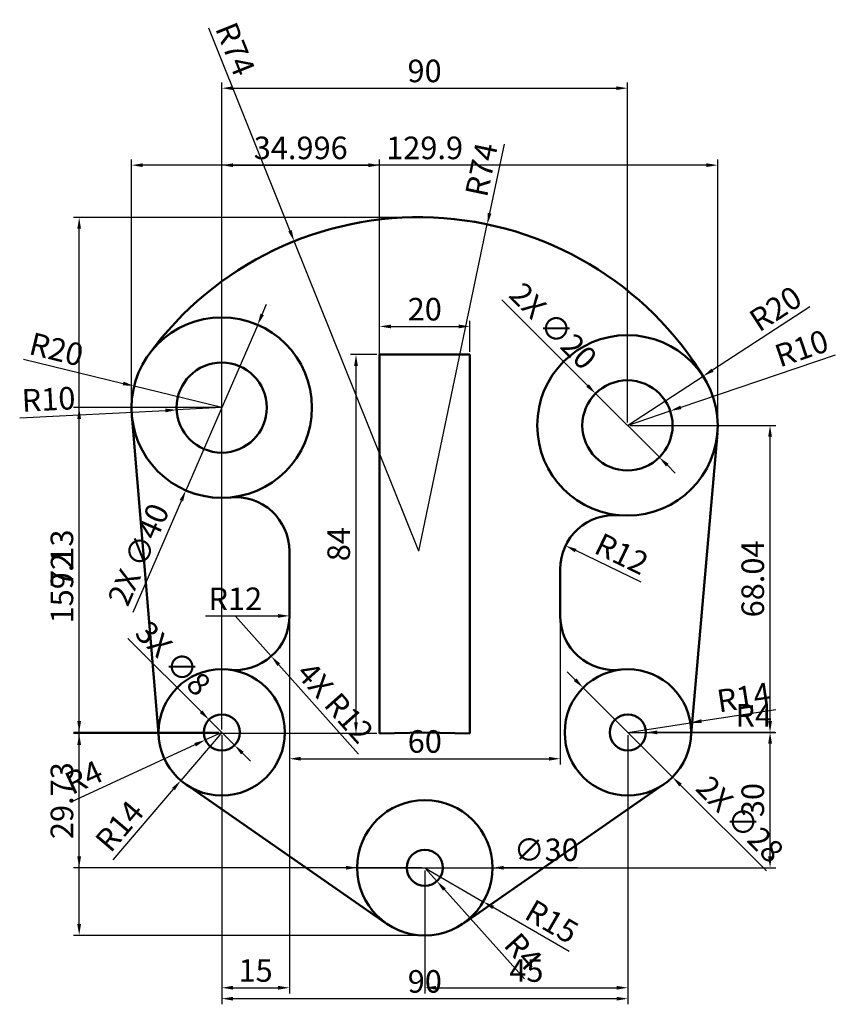
# Model space of a CAD drawing. Units: millimetres. Extents: x 2813 to 2994, y 1959 to 2178.
import ezdxf

# ---------------------------------------------------------------- set-up
doc = ezdxf.new("R2010")
doc.units = ezdxf.units.MM
doc.layers.add('M-DIMS', color=2, linetype='Continuous', lineweight=25)
doc.layers.add('M-OUTL', color=7, linetype='Continuous', lineweight=50)
doc.styles.get("Standard").update_dxf_attribs({"font": 'arial.ttf'})
doc.dimstyles.new('ISO-25', dxfattribs={"dimtxt": 5, "dimasz": 2.5, "dimexe": 1.25, "dimexo": 0.625, "dimtad": 1, "dimdec": 0, "dimtxsty": 'Standard', "dimcen": 2.5, "dimadec": 0, "dimazin": 0, "dimtfac": 1, "dimtdec": 0, "dimtmove": 0, "dimatfit": 3, "dimfxl": 1, "dimarcsym": 0})

# ---------------------------------------------------------------- blocks, each defined once
blk = doc.blocks.new('*D1')
at = {"layer": 'Defpoints', "color": 0, "transparency": 16777216}
for p in [(2847.97, 2091.08), (2857.96, 2091.6)]:
    blk.add_point(p, dxfattribs=at)
at = {"layer": 'M-DIMS', "color": 0, "lineweight": -2, "transparency": 16777216}
for p, q in [((2813.18, 2089.29), (2845.47, 2090.96)), ((2857.96, 2091.6), (2847.97, 2091.08))]:
    blk.add_line(p, q, dxfattribs=at)
at = {"layer": 'M-DIMS', "color": 0, "transparency": 16777216}
blk.add_solid([(2845.45, 2091.37), (2845.5, 2090.54), (2847.97, 2091.08)], dxfattribs=at)
at = {"layer": 'M-DIMS', "color": 0, "transparency": 16777216, "insert": (2819.6, 2092.8), "char_height": 5, "attachment_point": 5, "rotation": 2.9492}
blk.add_mtext('R10', dxfattribs=at)
blk = doc.blocks.new('*D2')
at = {"layer": 'Defpoints', "color": 0, "transparency": 16777216}
for p in [(2838.53, 2096.36), (2857.96, 2091.6)]:
    blk.add_point(p, dxfattribs=at)
at = {"layer": 'M-DIMS', "color": 0, "lineweight": -2, "transparency": 16777216}
for p, q in [((2814.01, 2102.36), (2836.1, 2096.95)), ((2857.96, 2091.6), (2838.53, 2096.36))]:
    blk.add_line(p, q, dxfattribs=at)
at = {"layer": 'M-DIMS', "color": 0, "transparency": 16777216}
blk.add_solid([(2836.2, 2097.36), (2836, 2096.55), (2838.53, 2096.36)], dxfattribs=at)
at = {"layer": 'M-DIMS', "color": 0, "transparency": 16777216, "insert": (2821.17, 2103.88), "char_height": 5, "attachment_point": 5, "rotation": 346.235}
blk.add_mtext('R20', dxfattribs=at)
blk = doc.blocks.new('*D3')
at = {"layer": 'Defpoints', "color": 0, "transparency": 16777216}
for p in [(2916.81, 2132.22), (2901.6, 2059.8)]:
    blk.add_point(p, dxfattribs=at)
at = {"layer": 'M-DIMS', "color": 0, "lineweight": -2, "transparency": 16777216}
for p, q in [((2920.55, 2150.01), (2917.33, 2134.67)), ((2901.6, 2059.8), (2916.81, 2132.22))]:
    blk.add_line(p, q, dxfattribs=at)
at = {"layer": 'M-DIMS', "color": 0, "transparency": 16777216}
blk.add_solid([(2916.92, 2134.75), (2917.73, 2134.58), (2916.81, 2132.22)], dxfattribs=at)
at = {"layer": 'M-DIMS', "color": 0, "transparency": 16777216, "insert": (2916.14, 2144.2), "char_height": 5, "attachment_point": 5, "rotation": 78.1387}
blk.add_mtext('R74', dxfattribs=at)
blk = doc.blocks.new('*D4')
at = {"layer": 'Defpoints', "color": 0, "transparency": 16777216}
for p in [(2964.64, 2098.54), (2947.87, 2087.64)]:
    blk.add_point(p, dxfattribs=at)
at = {"layer": 'M-DIMS', "color": 0, "lineweight": -2, "transparency": 16777216}
for p, q in [((2988.29, 2113.91), (2966.74, 2099.9)), ((2947.87, 2087.64), (2964.64, 2098.54))]:
    blk.add_line(p, q, dxfattribs=at)
at = {"layer": 'M-DIMS', "color": 0, "transparency": 16777216}
blk.add_solid([(2966.51, 2100.25), (2966.96, 2099.55), (2964.64, 2098.54)], dxfattribs=at)
at = {"layer": 'M-DIMS', "color": 0, "transparency": 16777216, "insert": (2981.03, 2112.98), "char_height": 5, "attachment_point": 5, "rotation": 33.0206}
blk.add_mtext('R20', dxfattribs=at)
blk = doc.blocks.new('*D5')
at = {"layer": 'Defpoints', "color": 0, "transparency": 16777216}
for p in [(2957.34, 2090.85), (2947.87, 2087.64)]:
    blk.add_point(p, dxfattribs=at)
at = {"layer": 'M-DIMS', "color": 0, "lineweight": -2, "transparency": 16777216}
for p, q in [((2993.94, 2103.24), (2959.71, 2091.65)), ((2947.87, 2087.64), (2957.34, 2090.85))]:
    blk.add_line(p, q, dxfattribs=at)
at = {"layer": 'M-DIMS', "color": 0, "transparency": 16777216}
blk.add_solid([(2959.58, 2092.04), (2959.84, 2091.26), (2957.34, 2090.85)], dxfattribs=at)
at = {"layer": 'M-DIMS', "color": 0, "transparency": 16777216, "insert": (2986.67, 2104.13), "char_height": 5, "attachment_point": 5, "rotation": 18.7049}
blk.add_mtext('R10', dxfattribs=at)
blk = doc.blocks.new('*D6')
at = {"layer": 'Defpoints', "color": 0, "transparency": 16777216}
for p in [(2934.15, 2060.98), (2944.96, 2055.77)]:
    blk.add_point(p, dxfattribs=at)
at = {"layer": 'M-DIMS', "color": 0, "lineweight": -2, "transparency": 16777216}
blk.add_line((2950.88, 2052.92), (2936.4, 2059.9), dxfattribs=at)
at = {"layer": 'M-DIMS', "color": 0, "transparency": 16777216}
blk.add_solid([(2936.58, 2060.27), (2936.22, 2059.52), (2934.15, 2060.98)], dxfattribs=at)
at = {"layer": 'M-DIMS', "color": 0, "transparency": 16777216, "insert": (2946.32, 2058.6), "char_height": 5, "attachment_point": 5, "rotation": 334.2857}
blk.add_mtext('R12', dxfattribs=at)
blk = doc.blocks.new('*D7')
at = {"layer": 'Defpoints', "color": 0, "transparency": 16777216}
for p in [(2961.8, 2021.72), (2947.96, 2019.6)]:
    blk.add_point(p, dxfattribs=at)
at = {"layer": 'M-DIMS', "color": 0, "lineweight": -2, "transparency": 16777216}
for p, q in [((2980.73, 2024.63), (2964.27, 2022.1)), ((2947.96, 2019.6), (2961.8, 2021.72))]:
    blk.add_line(p, q, dxfattribs=at)
at = {"layer": 'M-DIMS', "color": 0, "transparency": 16777216}
blk.add_solid([(2964.2, 2022.51), (2964.33, 2021.69), (2961.8, 2021.72)], dxfattribs=at)
at = {"layer": 'M-DIMS', "color": 0, "transparency": 16777216, "insert": (2973.74, 2026.73), "char_height": 5, "attachment_point": 5, "rotation": 8.72}
blk.add_mtext('R14', dxfattribs=at)
blk = doc.blocks.new('*D8')
at = {"layer": 'Defpoints', "color": 0, "transparency": 16777216}
for p in [(2947.96, 2019.6), (2951.96, 2019.6)]:
    blk.add_point(p, dxfattribs=at)
at = {"layer": 'M-DIMS', "color": 0, "lineweight": -2, "transparency": 16777216}
for p, q in [((2947.96, 2019.6), (2951.96, 2019.6)), ((2980.51, 2019.6), (2954.46, 2019.6))]:
    blk.add_line(p, q, dxfattribs=at)
at = {"layer": 'M-DIMS', "color": 0, "transparency": 16777216}
blk.add_solid([(2954.46, 2020.02), (2954.46, 2019.18), (2951.96, 2019.6)], dxfattribs=at)
at = {"layer": 'M-DIMS', "color": 0, "transparency": 16777216, "insert": (2975.86, 2022.72), "char_height": 5, "attachment_point": 5}
blk.add_mtext('R4', dxfattribs=at)
blk = doc.blocks.new('*D9')
at = {"layer": 'Defpoints', "color": 0, "transparency": 16777216}
for p in [(2902.96, 1989.6), (2915.93, 1982.07)]:
    blk.add_point(p, dxfattribs=at)
at = {"layer": 'M-DIMS', "color": 0, "lineweight": -2, "transparency": 16777216}
for p, q in [((2902.96, 1989.6), (2915.93, 1982.07)), ((2934.92, 1971.05), (2918.09, 1980.81))]:
    blk.add_line(p, q, dxfattribs=at)
at = {"layer": 'M-DIMS', "color": 0, "transparency": 16777216}
blk.add_solid([(2918.3, 1981.17), (2917.88, 1980.45), (2915.93, 1982.07)], dxfattribs=at)
at = {"layer": 'M-DIMS', "color": 0, "transparency": 16777216, "insert": (2930.79, 1977.12), "char_height": 5, "attachment_point": 5, "rotation": 329.8682}
blk.add_mtext('R15', dxfattribs=at)
blk = doc.blocks.new('*D10')
at = {"layer": 'Defpoints', "color": 0, "transparency": 16777216}
for p in [(2902.96, 1989.6), (2905.63, 1986.62)]:
    blk.add_point(p, dxfattribs=at)
at = {"layer": 'M-DIMS', "color": 0, "lineweight": -2, "transparency": 16777216}
for p, q in [((2902.96, 1989.6), (2905.63, 1986.62)), ((2925.07, 1965), (2907.3, 1984.77))]:
    blk.add_line(p, q, dxfattribs=at)
at = {"layer": 'M-DIMS', "color": 0, "transparency": 16777216}
blk.add_solid([(2907.61, 1985.04), (2906.99, 1984.49), (2905.63, 1986.62)], dxfattribs=at)
at = {"layer": 'M-DIMS', "color": 0, "transparency": 16777216, "insert": (2924.29, 1970.55), "char_height": 5, "attachment_point": 5, "rotation": 311.96}
blk.add_mtext('R4', dxfattribs=at)
blk = doc.blocks.new('*D11')
at = {"layer": 'Defpoints', "color": 0, "transparency": 16777216}
for p in [(2857.96, 2019.6), (2854.33, 2017.92)]:
    blk.add_point(p, dxfattribs=at)
at = {"layer": 'M-DIMS', "color": 0, "lineweight": -2, "transparency": 16777216}
for p, q in [((2857.96, 2019.6), (2854.33, 2017.92)), ((2824.74, 2004.28), (2852.06, 2016.88))]:
    blk.add_line(p, q, dxfattribs=at)
at = {"layer": 'M-DIMS', "color": 0, "transparency": 16777216}
blk.add_solid([(2851.88, 2017.25), (2852.23, 2016.5), (2854.33, 2017.92)], dxfattribs=at)
at = {"layer": 'M-DIMS', "color": 0, "transparency": 16777216, "insert": (2827.65, 2009.06), "char_height": 5, "attachment_point": 5, "rotation": 24.7633}
blk.add_mtext('R4', dxfattribs=at)
blk = doc.blocks.new('*D12')
at = {"layer": 'Defpoints', "color": 0, "transparency": 16777216}
for p in [(2857.96, 2019.6), (2848.88, 2008.94)]:
    blk.add_point(p, dxfattribs=at)
at = {"layer": 'M-DIMS', "color": 0, "lineweight": -2, "transparency": 16777216}
for p, q in [((2857.96, 2019.6), (2848.88, 2008.94)), ((2833.89, 1991.36), (2847.26, 2007.04))]:
    blk.add_line(p, q, dxfattribs=at)
at = {"layer": 'M-DIMS', "color": 0, "transparency": 16777216}
blk.add_solid([(2846.94, 2007.31), (2847.57, 2006.77), (2848.88, 2008.94)], dxfattribs=at)
at = {"layer": 'M-DIMS', "color": 0, "transparency": 16777216, "insert": (2835.78, 1998.41), "char_height": 5, "attachment_point": 5, "rotation": 49.5609}
blk.add_mtext('R14', dxfattribs=at)
blk = doc.blocks.new('*D13')
at = {"layer": 'Defpoints', "color": 0, "transparency": 16777216}
for p in [(2860.96, 2045.43), (2872.96, 2045.43)]:
    blk.add_point(p, dxfattribs=at)
at = {"layer": 'M-DIMS', "color": 0, "lineweight": -2, "transparency": 16777216}
blk.add_line((2854.38, 2045.43), (2870.46, 2045.43), dxfattribs=at)
blk.add_arc((2860.96, 2045.43), 12, 2.9842, 5.9683, dxfattribs=at)
at = {"layer": 'M-DIMS', "color": 0, "transparency": 16777216}
blk.add_solid([(2870.46, 2045.84), (2870.46, 2045.01), (2872.96, 2045.43)], dxfattribs=at)
at = {"layer": 'M-DIMS', "color": 0, "transparency": 16777216, "insert": (2860.96, 2048.56), "char_height": 5, "attachment_point": 5}
blk.add_mtext('R12', dxfattribs=at)
blk = doc.blocks.new('*D14')
at = {"layer": 'Defpoints', "color": 0, "transparency": 16777216}
for p in [(2857.96, 2019.6), (2947.96, 2019.6), (2947.96, 1960.58)]:
    blk.add_point(p, dxfattribs=at)
at = {"layer": 'M-DIMS', "color": 0, "lineweight": -2, "transparency": 16777216}
for p, q in [((2857.96, 2018.97), (2857.96, 1959.33)), ((2947.96, 2018.97), (2947.96, 1959.33)), ((2860.46, 1960.58), (2945.46, 1960.58))]:
    blk.add_line(p, q, dxfattribs=at)
at = {"layer": 'M-DIMS', "color": 0, "transparency": 16777216}
for points in [[(2860.46, 1960.99), (2860.46, 1960.16), (2857.96, 1960.58)], [(2945.46, 1960.99), (2945.46, 1960.16), (2947.96, 1960.58)]]:
    blk.add_solid(points, dxfattribs=at)
at = {"layer": 'M-DIMS', "color": 0, "transparency": 16777216, "insert": (2902.96, 1963.76), "char_height": 5, "attachment_point": 5}
blk.add_mtext('90', dxfattribs=at)
blk = doc.blocks.new('*D15')
at = {"layer": 'Defpoints', "color": 0, "transparency": 16777216}
for p in [(2947.87, 2162.39), (2857.96, 2091.6), (2947.87, 2087.64)]:
    blk.add_point(p, dxfattribs=at)
at = {"layer": 'M-DIMS', "color": 0, "lineweight": -2, "transparency": 16777216}
for p, q in [((2857.96, 2092.22), (2857.96, 2163.64)), ((2947.87, 2088.27), (2947.87, 2163.64)), ((2860.46, 2162.39), (2945.37, 2162.39))]:
    blk.add_line(p, q, dxfattribs=at)
at = {"layer": 'M-DIMS', "color": 0, "transparency": 16777216}
for points in [[(2860.46, 2162.81), (2860.46, 2161.98), (2857.96, 2162.39)], [(2945.37, 2162.81), (2945.37, 2161.98), (2947.87, 2162.39)]]:
    blk.add_solid(points, dxfattribs=at)
at = {"layer": 'M-DIMS', "color": 0, "transparency": 16777216, "insert": (2902.91, 2165.57), "char_height": 5, "attachment_point": 5}
blk.add_mtext('90', dxfattribs=at)
blk = doc.blocks.new('*D16')
at = {"layer": 'Defpoints', "color": 0, "transparency": 16777216}
for p in [(2892.95, 2103.33), (2887.71, 2019.33), (2892.95, 2019.33)]:
    blk.add_point(p, dxfattribs=at)
at = {"layer": 'M-DIMS', "color": 0, "lineweight": -2, "transparency": 16777216}
for p, q in [((2892.33, 2103.33), (2886.46, 2103.33)), ((2887.71, 2100.83), (2887.71, 2021.83)), ((2892.33, 2019.33), (2886.46, 2019.33))]:
    blk.add_line(p, q, dxfattribs=at)
at = {"layer": 'M-DIMS', "color": 0, "transparency": 16777216}
for points in [[(2887.29, 2100.83), (2888.12, 2100.83), (2887.71, 2103.33)], [(2887.29, 2021.83), (2888.12, 2021.83), (2887.71, 2019.33)]]:
    blk.add_solid(points, dxfattribs=at)
at = {"layer": 'M-DIMS', "color": 0, "transparency": 16777216, "insert": (2884.53, 2061.33), "char_height": 5, "attachment_point": 5, "rotation": 90}
blk.add_mtext('84', dxfattribs=at)
blk = doc.blocks.new('*D17')
at = {"layer": 'Defpoints', "color": 0, "transparency": 16777216}
for p in [(2912.95, 2109.58), (2892.95, 2103.33), (2912.95, 2103.33)]:
    blk.add_point(p, dxfattribs=at)
at = {"layer": 'M-DIMS', "color": 0, "lineweight": -2, "transparency": 16777216}
for p, q in [((2892.95, 2103.96), (2892.95, 2110.83)), ((2912.95, 2103.96), (2912.95, 2110.83)), ((2895.45, 2109.58), (2910.45, 2109.58))]:
    blk.add_line(p, q, dxfattribs=at)
at = {"layer": 'M-DIMS', "color": 0, "transparency": 16777216}
for points in [[(2895.45, 2110), (2895.45, 2109.16), (2892.95, 2109.58)], [(2910.45, 2110), (2910.45, 2109.16), (2912.95, 2109.58)]]:
    blk.add_solid(points, dxfattribs=at)
at = {"layer": 'M-DIMS', "color": 0, "transparency": 16777216, "insert": (2902.95, 2112.76), "char_height": 5, "attachment_point": 5}
blk.add_mtext('20', dxfattribs=at)
blk = doc.blocks.new('*D18')
at = {"layer": 'Defpoints', "color": 0, "transparency": 16777216}
for p in [(2872.96, 2045.43), (2932.96, 2045.43), (2932.96, 2013.76)]:
    blk.add_point(p, dxfattribs=at)
at = {"layer": 'M-DIMS', "color": 0, "lineweight": -2, "transparency": 16777216}
for p, q in [((2872.96, 2044.8), (2872.96, 2012.51)), ((2932.96, 2044.8), (2932.96, 2012.51)), ((2875.46, 2013.76), (2930.46, 2013.76))]:
    blk.add_line(p, q, dxfattribs=at)
at = {"layer": 'M-DIMS', "color": 0, "transparency": 16777216}
for points in [[(2875.46, 2014.18), (2875.46, 2013.34), (2872.96, 2013.76)], [(2930.46, 2014.18), (2930.46, 2013.34), (2932.96, 2013.76)]]:
    blk.add_solid(points, dxfattribs=at)
at = {"layer": 'M-DIMS', "color": 0, "transparency": 16777216, "insert": (2902.96, 2016.94), "char_height": 5, "attachment_point": 5}
blk.add_mtext('60', dxfattribs=at)
blk = doc.blocks.new('BOSS-OD40-BORE20')
for radius in [20, 10]:
    blk.add_circle((0, 0), radius)
blk = doc.blocks.new('BOSS-OD28-BORE8')
for radius in [14, 4]:
    blk.add_circle((0, 0), radius)
blk = doc.blocks.new('*D21')
at = {"layer": 'Defpoints', "color": 0, "transparency": 16777216}
for p in [(2837.96, 2145.33), (2837.96, 2091.6), (2967.87, 2087.64)]:
    blk.add_point(p, dxfattribs=at)
at = {"layer": 'M-DIMS', "color": 0, "lineweight": -2, "transparency": 16777216}
for p, q in [((2837.96, 2092.22), (2837.96, 2146.58)), ((2967.87, 2088.27), (2967.87, 2146.58)), ((2965.37, 2145.33), (2840.46, 2145.33))]:
    blk.add_line(p, q, dxfattribs=at)
at = {"layer": 'M-DIMS', "color": 0, "transparency": 16777216}
for points in [[(2840.46, 2145.74), (2840.46, 2144.91), (2837.96, 2145.33)], [(2965.37, 2145.74), (2965.37, 2144.91), (2967.87, 2145.33)]]:
    blk.add_solid(points, dxfattribs=at)
at = {"layer": 'M-DIMS', "color": 0, "transparency": 16777216, "insert": (2902.91, 2148.51), "char_height": 5, "attachment_point": 5}
blk.add_mtext('129.9', dxfattribs=at)
blk = doc.blocks.new('*D22')
at = {"layer": 'Defpoints', "color": 0, "transparency": 16777216}
for p in [(2826.36, 2133.73), (2904.86, 2133.73), (2902.96, 1974.6)]:
    blk.add_point(p, dxfattribs=at)
at = {"layer": 'M-DIMS', "color": 0, "lineweight": -2, "transparency": 16777216}
for p, q in [((2904.23, 2133.73), (2825.11, 2133.73)), ((2826.36, 1977.1), (2826.36, 2131.23)), ((2902.33, 1974.6), (2825.11, 1974.6))]:
    blk.add_line(p, q, dxfattribs=at)
at = {"layer": 'M-DIMS', "color": 0, "transparency": 16777216}
for points in [[(2825.94, 2131.23), (2826.77, 2131.23), (2826.36, 2133.73)], [(2825.94, 1977.1), (2826.77, 1977.1), (2826.36, 1974.6)]]:
    blk.add_solid(points, dxfattribs=at)
at = {"layer": 'M-DIMS', "color": 0, "transparency": 16777216, "insert": (2823.18, 2054.16), "char_height": 5, "attachment_point": 5, "rotation": 90}
blk.add_mtext('159.13', dxfattribs=at)
blk = doc.blocks.new('*D23')
at = {"layer": 'Defpoints', "color": 0, "transparency": 16777216}
for p in [(2826.36, 2091.6), (2857.96, 2091.6), (2857.96, 2019.6)]:
    blk.add_point(p, dxfattribs=at)
at = {"layer": 'M-DIMS', "color": 0, "lineweight": -2, "transparency": 16777216}
for p, q in [((2857.33, 2091.6), (2825.11, 2091.6)), ((2826.36, 2022.1), (2826.36, 2089.1)), ((2857.33, 2019.6), (2825.11, 2019.6))]:
    blk.add_line(p, q, dxfattribs=at)
at = {"layer": 'M-DIMS', "color": 0, "transparency": 16777216}
for points in [[(2825.94, 2089.1), (2826.77, 2089.1), (2826.36, 2091.6)], [(2825.94, 2022.1), (2826.77, 2022.1), (2826.36, 2019.6)]]:
    blk.add_solid(points, dxfattribs=at)
at = {"layer": 'M-DIMS', "color": 0, "transparency": 16777216, "insert": (2823.22, 2055.6), "char_height": 5, "attachment_point": 5, "rotation": 90}
blk.add_mtext('72', dxfattribs=at)
blk = doc.blocks.new('*D24')
at = {"layer": 'Defpoints', "color": 0, "transparency": 16777216}
for p in [(2947.87, 2087.64), (2979.47, 2087.64), (2947.96, 2019.6)]:
    blk.add_point(p, dxfattribs=at)
at = {"layer": 'M-DIMS', "color": 0, "lineweight": -2, "transparency": 16777216}
for p, q in [((2948.5, 2087.64), (2980.72, 2087.64)), ((2979.47, 2022.1), (2979.47, 2085.14)), ((2948.58, 2019.6), (2980.72, 2019.6))]:
    blk.add_line(p, q, dxfattribs=at)
at = {"layer": 'M-DIMS', "color": 0, "transparency": 16777216}
for points in [[(2979.05, 2085.14), (2979.89, 2085.14), (2979.47, 2087.64)], [(2979.05, 2022.1), (2979.89, 2022.1), (2979.47, 2019.6)]]:
    blk.add_solid(points, dxfattribs=at)
at = {"layer": 'M-DIMS', "color": 0, "transparency": 16777216, "insert": (2976.29, 2053.62), "char_height": 5, "attachment_point": 5, "rotation": 90}
blk.add_mtext('68.04', dxfattribs=at)
blk = doc.blocks.new('*D25')
at = {"layer": 'Defpoints', "color": 0, "transparency": 16777216}
for p in [(2947.96, 2019.6), (2979.47, 2019.6), (2902.96, 1989.6)]:
    blk.add_point(p, dxfattribs=at)
at = {"layer": 'M-DIMS', "color": 0, "lineweight": -2, "transparency": 16777216}
for p, q in [((2948.58, 2019.6), (2980.72, 2019.6)), ((2979.47, 1992.1), (2979.47, 2017.1)), ((2903.58, 1989.6), (2980.72, 1989.6))]:
    blk.add_line(p, q, dxfattribs=at)
at = {"layer": 'M-DIMS', "color": 0, "transparency": 16777216}
for points in [[(2979.05, 2017.1), (2979.89, 2017.1), (2979.47, 2019.6)], [(2979.05, 1992.1), (2979.89, 1992.1), (2979.47, 1989.6)]]:
    blk.add_solid(points, dxfattribs=at)
at = {"layer": 'M-DIMS', "color": 0, "transparency": 16777216, "insert": (2976.29, 2004.6), "char_height": 5, "attachment_point": 5, "rotation": 90}
blk.add_mtext('30', dxfattribs=at)
blk = doc.blocks.new('*D26')
at = {"layer": 'Defpoints', "color": 0, "transparency": 16777216}
for p in [(2947.96, 2019.6), (2902.96, 1989.6), (2947.96, 1963)]:
    blk.add_point(p, dxfattribs=at)
at = {"layer": 'M-DIMS', "color": 0, "lineweight": -2, "transparency": 16777216}
for p, q in [((2947.96, 2018.97), (2947.96, 1961.75)), ((2902.96, 1988.97), (2902.96, 1961.75)), ((2905.46, 1963), (2945.46, 1963))]:
    blk.add_line(p, q, dxfattribs=at)
at = {"layer": 'M-DIMS', "color": 0, "transparency": 16777216}
for points in [[(2905.46, 1963.42), (2905.46, 1962.58), (2902.96, 1963)], [(2945.46, 1963.42), (2945.46, 1962.58), (2947.96, 1963)]]:
    blk.add_solid(points, dxfattribs=at)
at = {"layer": 'M-DIMS', "color": 0, "transparency": 16777216, "insert": (2925.46, 1966.17), "char_height": 5, "attachment_point": 5}
blk.add_mtext('45', dxfattribs=at)
blk = doc.blocks.new('*D27')
at = {"layer": 'Defpoints', "color": 0, "transparency": 16777216}
for p in [(2892.95, 2145.33), (2857.96, 2019.6), (2892.95, 2019.33)]:
    blk.add_point(p, dxfattribs=at)
at = {"layer": 'M-DIMS', "color": 0, "lineweight": -2, "transparency": 16777216}
for p, q in [((2857.96, 2020.22), (2857.96, 2146.58)), ((2892.95, 2019.96), (2892.95, 2146.58)), ((2860.46, 2145.33), (2890.45, 2145.33))]:
    blk.add_line(p, q, dxfattribs=at)
at = {"layer": 'M-DIMS', "color": 0, "transparency": 16777216}
for points in [[(2860.46, 2145.74), (2860.46, 2144.91), (2857.96, 2145.33)], [(2890.45, 2145.74), (2890.45, 2144.91), (2892.95, 2145.33)]]:
    blk.add_solid(points, dxfattribs=at)
at = {"layer": 'M-DIMS', "color": 0, "transparency": 16777216, "insert": (2875.46, 2148.51), "char_height": 5, "attachment_point": 5}
blk.add_mtext('34.996', dxfattribs=at)
blk = doc.blocks.new('*D28')
at = {"layer": 'Defpoints', "color": 0, "transparency": 16777216}
for p in [(2826.36, 2019.33), (2892.95, 2019.33), (2902.96, 1989.6)]:
    blk.add_point(p, dxfattribs=at)
at = {"layer": 'M-DIMS', "color": 0, "lineweight": -2, "transparency": 16777216}
for p, q in [((2892.33, 2019.33), (2825.11, 2019.33)), ((2826.36, 1992.1), (2826.36, 2016.83)), ((2902.33, 1989.6), (2825.11, 1989.6))]:
    blk.add_line(p, q, dxfattribs=at)
at = {"layer": 'M-DIMS', "color": 0, "transparency": 16777216}
for points in [[(2825.94, 2016.83), (2826.77, 2016.83), (2826.36, 2019.33)], [(2825.94, 1992.1), (2826.77, 1992.1), (2826.36, 1989.6)]]:
    blk.add_solid(points, dxfattribs=at)
at = {"layer": 'M-DIMS', "color": 0, "transparency": 16777216, "insert": (2823.18, 2004.47), "char_height": 5, "attachment_point": 5, "rotation": 90}
blk.add_mtext('29.73', dxfattribs=at)
blk = doc.blocks.new('*D29')
at = {"layer": 'Defpoints', "color": 0, "transparency": 16777216}
for p in [(2872.96, 2045.43), (2857.96, 2019.6), (2872.96, 1963)]:
    blk.add_point(p, dxfattribs=at)
at = {"layer": 'M-DIMS', "color": 0, "lineweight": -2, "transparency": 16777216}
for p, q in [((2872.96, 2044.8), (2872.96, 1961.75)), ((2857.96, 2018.97), (2857.96, 1961.75)), ((2860.46, 1963), (2870.46, 1963))]:
    blk.add_line(p, q, dxfattribs=at)
at = {"layer": 'M-DIMS', "color": 0, "transparency": 16777216}
for points in [[(2860.46, 1963.42), (2860.46, 1962.58), (2857.96, 1963)], [(2870.46, 1963.42), (2870.46, 1962.58), (2872.96, 1963)]]:
    blk.add_solid(points, dxfattribs=at)
at = {"layer": 'M-DIMS', "color": 0, "transparency": 16777216, "insert": (2865.46, 1966.18), "char_height": 5, "attachment_point": 5}
blk.add_mtext('15', dxfattribs=at)
blk = doc.blocks.new('*D30')
at = {"layer": 'Defpoints', "color": 0, "transparency": 16777216}
for p in [(2874.01, 2128.46), (2901.6, 2059.8)]:
    blk.add_point(p, dxfattribs=at)
at = {"layer": 'M-DIMS', "color": 0, "lineweight": -2, "transparency": 16777216}
for p, q in [((2855.01, 2175.78), (2873.08, 2130.78)), ((2901.6, 2059.8), (2874.01, 2128.46))]:
    blk.add_line(p, q, dxfattribs=at)
at = {"layer": 'M-DIMS', "color": 0, "transparency": 16777216}
blk.add_solid([(2873.47, 2130.94), (2872.7, 2130.63), (2874.01, 2128.46)], dxfattribs=at)
at = {"layer": 'M-DIMS', "color": 0, "transparency": 16777216, "insert": (2860.36, 2170.83), "char_height": 5, "attachment_point": 5, "rotation": 291.8887}
blk.add_mtext('R74', dxfattribs=at)
blk = doc.blocks.new('*D31')
at = {"layer": 'Defpoints', "color": 0, "transparency": 16777216}
for p in [(2865.92, 2109.95), (2850, 2073.25)]:
    blk.add_point(p, dxfattribs=at)
at = {"layer": 'M-DIMS', "color": 0, "lineweight": -2, "transparency": 16777216}
for p, q in [((2866.91, 2112.24), (2867.91, 2114.53)), ((2865.92, 2109.95), (2850, 2073.25)), ((2838.3, 2046.28), (2849.01, 2070.96))]:
    blk.add_line(p, q, dxfattribs=at)
at = {"layer": 'M-DIMS', "color": 0, "transparency": 16777216}
for points in [[(2866.53, 2112.41), (2867.29, 2112.08), (2865.92, 2109.95)], [(2848.62, 2071.12), (2849.39, 2070.79), (2850, 2073.25)]]:
    blk.add_solid(points, dxfattribs=at)
at = {"layer": 'M-DIMS', "color": 0, "transparency": 16777216, "insert": (2840.11, 2058.79), "char_height": 5, "attachment_point": 5, "rotation": 66.5538}
blk.add_mtext('2X ∅40', dxfattribs=at)
blk = doc.blocks.new('*D32')
at = {"layer": 'Defpoints', "color": 0, "transparency": 16777216}
for p in [(2940.8, 2094.71), (2954.94, 2080.57)]:
    blk.add_point(p, dxfattribs=at)
at = {"layer": 'M-DIMS', "color": 0, "lineweight": -2, "transparency": 16777216}
for p, q in [((2920.01, 2115.5), (2939.03, 2096.48)), ((2954.94, 2080.57), (2940.8, 2094.71)), ((2956.71, 2078.8), (2958.48, 2077.04))]:
    blk.add_line(p, q, dxfattribs=at)
at = {"layer": 'M-DIMS', "color": 0, "transparency": 16777216}
for points in [[(2939.33, 2096.77), (2938.74, 2096.18), (2940.8, 2094.71)], [(2957.01, 2079.1), (2956.42, 2078.51), (2954.94, 2080.57)]]:
    blk.add_solid(points, dxfattribs=at)
at = {"layer": 'M-DIMS', "color": 0, "transparency": 16777216, "insert": (2930.98, 2109.22), "char_height": 5, "attachment_point": 5, "rotation": 315.0088}
blk.add_mtext('2X ∅20', dxfattribs=at)
blk = doc.blocks.new('*D33')
at = {"layer": 'Defpoints', "color": 0, "transparency": 16777216}
for p in [(2887.96, 1989.6), (2917.96, 1989.6)]:
    blk.add_point(p, dxfattribs=at)
at = {"layer": 'M-DIMS', "color": 0, "lineweight": -2, "transparency": 16777216}
for p, q in [((2885.46, 1989.6), (2882.96, 1989.6)), ((2887.96, 1989.6), (2917.96, 1989.6)), ((2936.79, 1989.6), (2920.46, 1989.6))]:
    blk.add_line(p, q, dxfattribs=at)
at = {"layer": 'M-DIMS', "color": 0, "transparency": 16777216}
for points in [[(2885.46, 1990.02), (2885.46, 1989.18), (2887.96, 1989.6)], [(2920.46, 1990.02), (2920.46, 1989.18), (2917.96, 1989.6)]]:
    blk.add_solid(points, dxfattribs=at)
at = {"layer": 'M-DIMS', "color": 0, "transparency": 16777216, "insert": (2929.88, 1992.92), "char_height": 5, "attachment_point": 5, "rotation": 0}
blk.add_mtext('∅30', dxfattribs=at)
blk = doc.blocks.new('*D34')
at = {"layer": 'Defpoints', "color": 0, "transparency": 16777216}
for p in [(2938.06, 2029.5), (2957.86, 2009.7)]:
    blk.add_point(p, dxfattribs=at)
at = {"layer": 'M-DIMS', "color": 0, "lineweight": -2, "transparency": 16777216}
for p, q in [((2936.29, 2031.26), (2934.52, 2033.03)), ((2938.06, 2029.5), (2957.86, 2009.7)), ((2978.67, 1988.9), (2959.63, 2007.93))]:
    blk.add_line(p, q, dxfattribs=at)
at = {"layer": 'M-DIMS', "color": 0, "transparency": 16777216}
for points in [[(2936.58, 2031.56), (2935.99, 2030.97), (2938.06, 2029.5)], [(2959.92, 2008.23), (2959.33, 2007.64), (2957.86, 2009.7)]]:
    blk.add_solid(points, dxfattribs=at)
at = {"layer": 'M-DIMS', "color": 0, "transparency": 16777216, "insert": (2972.38, 1999.88), "char_height": 5, "attachment_point": 5, "rotation": 315.009}
blk.add_mtext('2X ∅28', dxfattribs=at)
blk = doc.blocks.new('*D35')
at = {"layer": 'Defpoints', "color": 0, "transparency": 16777216}
for p in [(2855.13, 2022.43), (2860.78, 2016.77)]:
    blk.add_point(p, dxfattribs=at)
at = {"layer": 'M-DIMS', "color": 0, "lineweight": -2, "transparency": 16777216}
for p, q in [((2837.14, 2040.44), (2853.36, 2024.2)), ((2860.78, 2016.77), (2855.13, 2022.43)), ((2862.55, 2015), (2864.32, 2013.23))]:
    blk.add_line(p, q, dxfattribs=at)
at = {"layer": 'M-DIMS', "color": 0, "transparency": 16777216}
for points in [[(2853.66, 2024.49), (2853.07, 2023.9), (2855.13, 2022.43)], [(2862.85, 2015.29), (2862.26, 2014.71), (2860.78, 2016.77)]]:
    blk.add_solid(points, dxfattribs=at)
at = {"layer": 'M-DIMS', "color": 0, "transparency": 16777216, "insert": (2846.72, 2035.55), "char_height": 5, "attachment_point": 5, "rotation": 314.9685}
blk.add_mtext('3X ∅8', dxfattribs=at)
blk = doc.blocks.new('*D36')
at = {"layer": 'Defpoints', "color": 0, "transparency": 16777216}
for p in [(2860.96, 2045.43), (2868.94, 2036.46)]:
    blk.add_point(p, dxfattribs=at)
at = {"layer": 'M-DIMS', "color": 0, "lineweight": -2, "transparency": 16777216}
for p, q in [((2860.96, 2045.43), (2868.94, 2036.46)), ((2888.29, 2014.74), (2870.6, 2034.6))]:
    blk.add_line(p, q, dxfattribs=at)
at = {"layer": 'M-DIMS', "color": 0, "transparency": 16777216}
blk.add_solid([(2870.91, 2034.87), (2870.29, 2034.32), (2868.94, 2036.46)], dxfattribs=at)
at = {"layer": 'M-DIMS', "color": 0, "transparency": 16777216, "insert": (2882.62, 2025.82), "char_height": 5, "attachment_point": 5, "rotation": 311.6887}
blk.add_mtext('4X R12', dxfattribs=at)

msp = doc.modelspace()

# ---------------------------------------------------------------- linework, layer by layer
at = {"layer": 'M-OUTL'}
for p, q in [((2912.9543, 2103.3314), (2892.9543, 2103.3314)), ((2892.9543, 2103.3314), (2892.9543, 2019.3314)), ((2912.9543, 2019.3314), (2912.9543, 2103.3314)), ((2844.0066, 2018.4323), (2838.0275, 2089.9323)), ((2961.9049, 2018.3823), (2967.7952, 2085.9032)), ((2872.9579, 2045.4253), (2872.9579, 2059.7399)), ((2932.9579, 2045.4253), (2932.9579, 2055.7742)), ((2892.9543, 2019.3314), (2902.9579, 2019.599)), ((2902.9579, 2019.599), (2912.9543, 2019.3314)), ((2894.408, 1977.2742), (2849.978, 2008.0959)), ((2911.5077, 1977.2742), (2955.9378, 2008.0959))]:
    msp.add_line(p, q, dxfattribs=at)
for radius in [15, 4]:
    msp.add_circle((2902.9579, 1989.599), radius, dxfattribs=at)
for centre, radius, start, end in [((2901.6018, 2059.7994), 74, 31.036966, 143.922347), ((2860.9579, 2059.7399), 12, 0, 95.379379), ((2944.9579, 2055.7742), 12, 84.77717, 180), ((2860.9579, 2045.4253), 12, 263.37419, 0), ((2944.9579, 2045.4253), 12, 180, 276.62581)]:
    msp.add_arc(centre, radius, start, end, dxfattribs=at)

# ---------------------------------------------------------------- block references
for name, p in [('BOSS-OD40-BORE20', (2857.9579, 2091.599)), ('BOSS-OD40-BORE20', (2947.8708, 2087.6413)), ('BOSS-OD28-BORE8', (2857.9579, 2019.599)), ('BOSS-OD28-BORE8', (2947.9579, 2019.599))]:
    msp.add_blockref(name, p, dxfattribs=at)

# ---------------------------------------------------------------- dimensions: what is measured, and where the dimension line sits
at = {"layer": 'M-DIMS'}
for center, mpoint, override, picture, middle in [((2901.6018, 2059.7994), (2874.0142, 2128.4647), {"dimdec": 0, "dimlfac": 1, "dimrnd": 0, "dimzin": 0, "dimdsep": 46, "dimlunit": 2}, '*D30', (2857.4616, 2169.6639)), ((2947.8708, 2087.6413), (2964.6403, 2098.5401), {"dimclrd": 0, "dimclre": 0, "dimclrt": 0}, '*D4', (2982.7638, 2110.3189)), ((2857.9579, 2091.599), (2838.5323, 2096.3578), {"dimclrd": 0, "dimclre": 0, "dimclrt": 0}, '*D2', (2820.4158, 2100.7959)), ((2947.8708, 2087.6413), (2957.3427, 2090.8483), {"dimclrd": 0, "dimclre": 0, "dimclrt": 0}, '*D5', (2987.6934, 2101.1243)), ((2857.9579, 2091.599), (2847.9711, 2091.0845), {"dimclrd": 0, "dimclre": 0, "dimclrt": 0}, '*D1', (2819.7586, 2089.631)), ((2944.9579, 2055.7742), (2934.1463, 2060.9808), {"dimclrd": 0, "dimclre": 0, "dimclrt": 0}, '*D6', (2944.9579, 2055.7742)), ((2860.9579, 2045.4253), (2872.9579, 2045.4253), {"dimclrd": 0, "dimclre": 0, "dimclrt": 0}, '*D13', (2860.9579, 2045.4253)), ((2947.9579, 2019.599), (2961.7961, 2021.7215), {"dimclrd": 0, "dimclre": 0, "dimclrt": 0}, '*D7', (2974.2192, 2023.6269)), ((2947.9579, 2019.599), (2951.9579, 2019.599), {"dimclrd": 0, "dimclre": 0, "dimclrt": 0}, '*D8', (2975.8624, 2019.599)), ((2857.9579, 2019.599), (2854.3257, 2017.9235), {"dimclrd": 0, "dimclre": 0, "dimclrt": 0}, '*D11', (2828.9605, 2006.2228)), ((2857.9579, 2019.599), (2848.8769, 2008.9436), {"dimclrd": 0, "dimclre": 0, "dimclrt": 0}, '*D12', (2838.1624, 1996.3715)), ((2902.9579, 1989.599), (2915.931, 1982.0691), {"dimclrd": 0, "dimclre": 0, "dimclrt": 0}, '*D9', (2929.1956, 1974.3701)), ((2902.9579, 1989.599), (2905.6323, 1986.6245), {"dimclrd": 0, "dimclre": 0, "dimclrt": 0}, '*D10', (2921.9655, 1968.4593))]:
    dim = msp.add_radius_dim(center=center, mpoint=mpoint, dimstyle='ISO-25', override=override, dxfattribs=at)
    dim.commit()
    dim.dimension.update_dxf_attribs({"geometry": picture, "text_midpoint": middle, "dimtype": 164})
for base, p1, p2, override, picture, middle in [((2947.8708, 2162.3933), (2857.9579, 2091.599), (2947.8708, 2087.6413), {"dimclrd": 0, "dimclre": 0, "dimclrt": 0}, '*D15', (2902.9144, 2165.5711)), ((2837.9579, 2145.3278), (2967.8708, 2087.6413), (2837.9579, 2091.599), {"dimdec": 1, "dimlfac": 1, "dimrnd": 0, "dimzin": 0, "dimdsep": 46, "dimlunit": 2}, '*D21', (2902.9144, 2148.5057)), ((2892.9543, 2145.3278), (2857.9579, 2019.599), (2892.9543, 2019.3314), {"dimdec": 3, "dimlfac": 1, "dimrnd": 0, "dimzin": 0, "dimdsep": 46, "dimlunit": 2}, '*D27', (2875.4561, 2148.5074)), ((2912.9543, 2109.5786), (2892.9543, 2103.3314), (2912.9543, 2103.3314), {"dimclrd": 0, "dimclre": 0, "dimclrt": 0}, '*D17', (2902.9543, 2112.7565)), ((2872.9579, 1962.999), (2857.9579, 2019.599), (2872.9579, 2045.4253), {"dimdec": 0, "dimlfac": 1, "dimrnd": 0, "dimzin": 0, "dimdsep": 46, "dimlunit": 2}, '*D29', (2865.4579, 1966.1769)), ((2932.9579, 2013.7616), (2872.9579, 2045.4253), (2932.9579, 2045.4253), {"dimclrd": 0, "dimclre": 0, "dimclrt": 0}, '*D18', (2902.9579, 2016.9395)), ((2947.9579, 1960.5782), (2857.9579, 2019.599), (2947.9579, 2019.599), {"dimclrd": 0, "dimclre": 0, "dimclrt": 0}, '*D14', (2902.9579, 1963.7561)), ((2947.9579, 1962.999), (2902.9579, 1989.599), (2947.9579, 2019.599), {"dimdec": 0, "dimlfac": 1, "dimrnd": 0, "dimzin": 0, "dimdsep": 46, "dimlunit": 2}, '*D26', (2925.4579, 1966.1666))]:
    dim = msp.add_linear_dim(base=base, p1=p1, p2=p2, dimstyle='ISO-25', override=override, dxfattribs=at)
    dim.commit()
    dim.dimension.update_dxf_attribs({"geometry": picture, "text_midpoint": middle})
dim = msp.add_radius_dim(center=(2901.6018, 2059.7994), mpoint=(2916.812, 2132.2194), dimstyle='ISO-25', override={"dimclrd": 0, "dimclre": 0, "dimclrt": 0}, dxfattribs=at)
dim.commit()
dim.dimension.update_dxf_attribs({"geometry": '*D3', "text_midpoint": (2916.1356, 2144.2028)})
for base, p1, p2, override, picture, middle in [((2826.3579, 2133.7278), (2902.9579, 1974.599), (2904.8558, 2133.7278), {"dimdec": 2, "dimlfac": 1, "dimrnd": 0, "dimzin": 0, "dimdsep": 46, "dimlunit": 2}, '*D22', (2823.1783, 2054.1634)), ((2887.7054, 2019.3314), (2892.9543, 2103.3314), (2892.9543, 2019.3314), {"dimclrd": 0, "dimclre": 0, "dimclrt": 0}, '*D16', (2884.5276, 2061.3314)), ((2826.3579, 2091.599), (2857.9579, 2019.599), (2857.9579, 2091.599), {"dimdec": 0, "dimlfac": 1, "dimrnd": 0, "dimzin": 0, "dimdsep": 46, "dimlunit": 2}, '*D23', (2823.2227, 2055.599)), ((2979.4708, 2087.6413), (2947.9579, 2019.599), (2947.8708, 2087.6413), {"dimdec": 2, "dimlfac": 1, "dimrnd": 0, "dimzin": 0, "dimdsep": 46, "dimlunit": 2}, '*D24', (2976.293, 2053.6202)), ((2826.3579, 2019.3314), (2902.9579, 1989.599), (2892.9543, 2019.3314), {"dimdec": 2, "dimlfac": 1, "dimrnd": 0, "dimzin": 0, "dimdsep": 46, "dimlunit": 2}, '*D28', (2823.1783, 2004.4652)), ((2979.4708, 2019.599), (2902.9579, 1989.599), (2947.9579, 2019.599), {"dimdec": 0, "dimlfac": 1, "dimrnd": 0, "dimzin": 0, "dimdsep": 46, "dimlunit": 2}, '*D25', (2976.2913, 2004.599))]:
    dim = msp.add_linear_dim(base=base, p1=p1, p2=p2, angle=90, dimstyle='ISO-25', override=override, dxfattribs=at)
    dim.commit()
    dim.dimension.update_dxf_attribs({"geometry": picture, "text_midpoint": middle})
for p1, p2, text, picture, middle in [((2954.943, 2080.5713), (2940.7987, 2094.7113), '2X <>', '*D32', (2928.6353, 2106.871)), ((2860.7848, 2016.769), (2855.131, 2022.429), '3X <>', '*D35', (2844.3706, 2033.2013)), ((2938.0569, 2029.4969), (2957.8589, 2009.7011), '2X <>', '*D34', (2970.032, 1997.5318))]:
    dim = msp.add_diameter_dim_2p(p1=p1, p2=p2, text=text, dimstyle='ISO-25', override={"dimdec": 0, "dimlfac": 1, "dimrnd": 0, "dimzin": 0, "dimdsep": 46, "dimlunit": 2}, dxfattribs=at)
    dim.commit()
    dim.dimension.update_dxf_attribs({"geometry": picture, "text_midpoint": middle, "dimtype": 163})
dim = msp.add_diameter_dim_2p(p1=(2865.9157, 2109.9477), p2=(2850.0001, 2073.2503), text='2X <>', dimstyle='ISO-25', override={"dimdec": 0, "dimlfac": 1, "dimrnd": 0, "dimzin": 0, "dimdsep": 46, "dimlunit": 2}, dxfattribs=at)
dim.commit()
dim.dimension.update_dxf_attribs({"geometry": '*D31', "text_midpoint": (2843.1569, 2057.4714)})
dim = msp.add_radius_dim(center=(2860.9579, 2045.4253), mpoint=(2868.9389, 2036.4641), text='4X <>', dimstyle='ISO-25', override={"dimdec": 0, "dimlfac": 1, "dimrnd": 0, "dimzin": 0, "dimdsep": 46, "dimlunit": 2}, dxfattribs=at)
dim.commit()
dim.dimension.update_dxf_attribs({"geometry": '*D36', "text_midpoint": (2882.6182, 2025.8214)})
dim = msp.add_diameter_dim_2p(p1=(2887.9579, 1989.599), p2=(2917.9579, 1989.599), dimstyle='ISO-25', override={"dimdec": 0, "dimlfac": 1, "dimrnd": 0, "dimzin": 0, "dimdsep": 46, "dimlunit": 2}, dxfattribs=at)
dim.commit()
dim.dimension.update_dxf_attribs({"geometry": '*D33', "text_midpoint": (2929.8755, 1989.599), "dimtype": 163})

doc.saveas('drawing.dxf')
